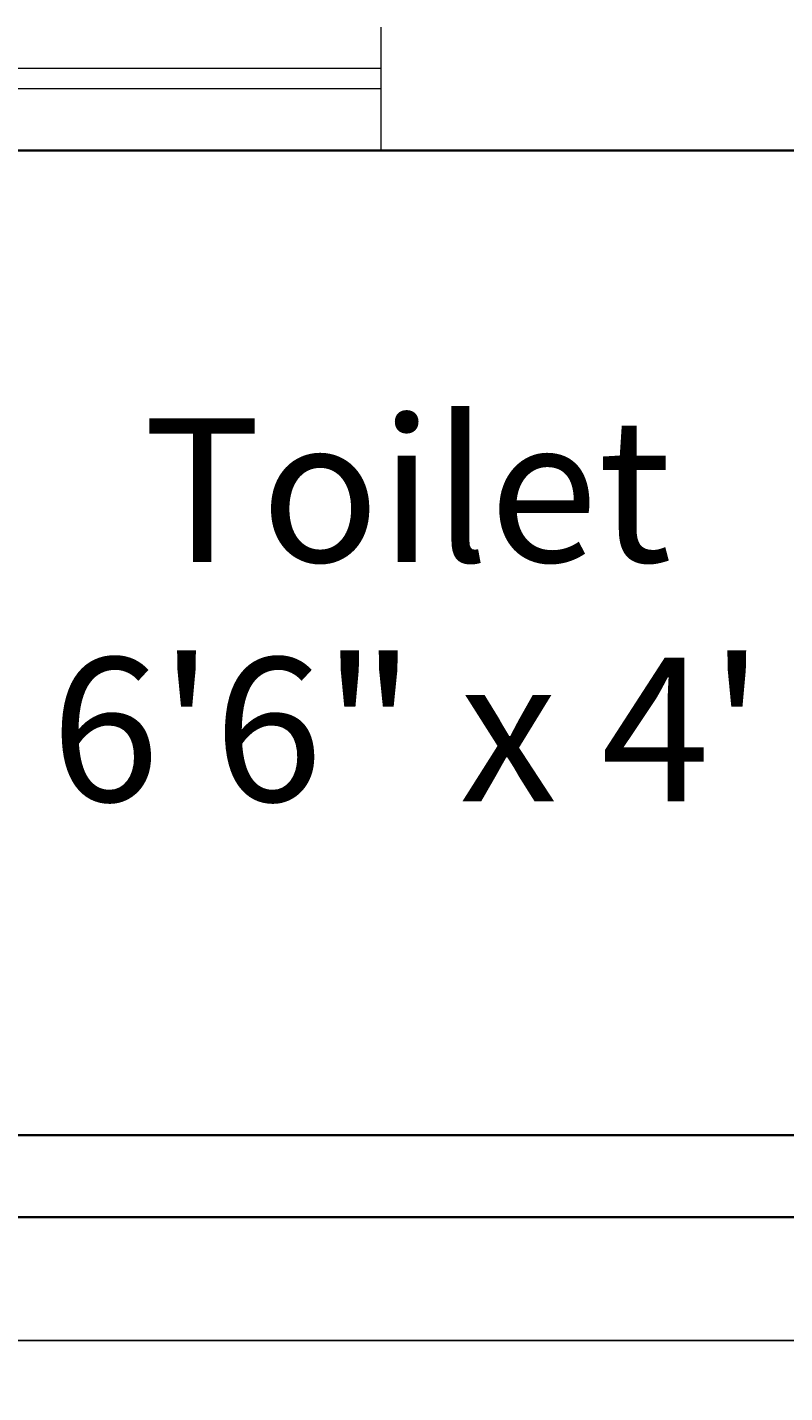
# Model space of a CAD drawing. Units: feet. Extents: x 105 to 1094, y -88 to 588.
# Tile 9 of 59: x 324 to 361, y 138 to 204. Entities that reach past the tile are written whole.
import ezdxf

# ---------------------------------------------------------------- set-up
doc = ezdxf.new("R2010")
doc.units = ezdxf.units.FT
doc.header["$MEASUREMENT"] = 0
for name, color, linetype, lineweight in [('A-ANNO-DIMS', 2, 'Continuous', 18), ('A-AREA-IDEN', 7, 'Continuous', 18), ('A-GLAZ', 4, 'Continuous', 18), ('A-WALL', 7, 'Continuous', 35)]:
    doc.layers.add(name, color=color, linetype=linetype, lineweight=lineweight)
doc.styles.get("Standard").update_dxf_attribs({"font": 'arial.ttf'})
doc.dimstyles.get("Standard").update_dxf_attribs({"dimtxt": 0.18, "dimasz": 0.18, "dimexe": 0.18, "dimexo": 0.0625, "dimgap": 0.09, "dimtad": 0, "dimtih": 1, "dimtoh": 1, "dimdec": 4, "dimzin": 0, "dimdsep": 46, "dimtxsty": 'Standard', "dimcen": 0.09, "dimadec": 0, "dimazin": 0, "dimtfac": 1, "dimtdec": 4, "dimtofl": 0, "dimtmove": 0, "dimatfit": 3, "dimfxl": 1, "dimtolj": 1, "dimtzin": 0, "dimarcsym": 0})

# ---------------------------------------------------------------- blocks, each defined once
blk = doc.blocks.new('VENT-TRANSVERSE')
for p, q in [((0, 0), (0, 6)), ((18, 0), (18, 6)), ((0, 3), (18, 3)), ((0, 2), (18, 2))]:
    blk.add_line(p, q)
blk = doc.blocks.new('*D20')
at = {"layer": 'A-ANNO-DIMS', "color": 0, "lineweight": -2, "transparency": 16777216}
for p, q in [((150.688, 276.019), (150.688, -88.149)), ((1048.688, 276.019), (1048.688, -88.149)), ((150.868, -87.969), (599.399, -87.969)), ((1048.508, -87.969), (599.977, -87.969))]:
    blk.add_line(p, q, dxfattribs=at)
at = {"layer": 'A-ANNO-DIMS', "color": 0, "transparency": 16777216}
for points in [[(150.868, -87.939), (150.868, -87.999), (150.688, -87.969)], [(1048.508, -87.939), (1048.508, -87.999), (1048.688, -87.969)]]:
    blk.add_solid(points, dxfattribs=at)
at = {"layer": 'Defpoints', "color": 0, "transparency": 16777216}
for p in [(150.688, 276.081), (1048.688, 276.081), (1048.688, -87.969)]:
    blk.add_point(p, dxfattribs=at)
at = {"layer": 'A-ANNO-DIMS', "color": 0, "transparency": 16777216, "insert": (599.688, -87.969), "char_height": 0.18, "attachment_point": 5}
blk.add_mtext('\\A1;898', dxfattribs=at)
blk = doc.blocks.new('*D21')
at = {"layer": 'A-ANNO-DIMS', "color": 0, "lineweight": -2, "transparency": 16777216}
for p, q in [((849.626, 543.081), (105.458, 543.081)), ((105.638, 542.901), (105.638, 250.263)), ((105.638, -42.739), (105.638, 249.899)), ((849.626, -42.919), (105.458, -42.919))]:
    blk.add_line(p, q, dxfattribs=at)
at = {"layer": 'A-ANNO-DIMS', "color": 0, "transparency": 16777216}
for points in [[(105.608, 542.901), (105.668, 542.901), (105.638, 543.081)], [(105.608, -42.739), (105.668, -42.739), (105.638, -42.919)]]:
    blk.add_solid(points, dxfattribs=at)
at = {"layer": 'Defpoints', "color": 0, "transparency": 16777216}
for p in [(105.638, 543.081), (849.688, 543.081), (849.688, -42.919)]:
    blk.add_point(p, dxfattribs=at)
at = {"layer": 'A-ANNO-DIMS', "color": 0, "transparency": 16777216, "insert": (105.638, 250.081), "char_height": 0.18, "attachment_point": 5}
blk.add_mtext('\\A1;586', dxfattribs=at)
blk = doc.blocks.new('*D39')
at = {"layer": 'A-ANNO-DIMS', "color": 0, "lineweight": -2, "transparency": 16777216}
for p, q in [((294.688, 204.144), (294.688, 588.311)), ((370.688, 204.144), (370.688, 588.311)), ((294.868, 588.131), (332.47, 588.131)), ((370.508, 588.131), (332.906, 588.131))]:
    blk.add_line(p, q, dxfattribs=at)
at = {"layer": 'A-ANNO-DIMS', "color": 0, "transparency": 16777216}
for points in [[(294.868, 588.161), (294.868, 588.101), (294.688, 588.131)], [(370.508, 588.161), (370.508, 588.101), (370.688, 588.131)]]:
    blk.add_solid(points, dxfattribs=at)
at = {"layer": 'Defpoints', "color": 0, "transparency": 16777216}
for p in [(370.688, 588.131), (294.688, 204.081), (370.688, 204.081)]:
    blk.add_point(p, dxfattribs=at)
at = {"layer": 'A-ANNO-DIMS', "color": 0, "transparency": 16777216, "insert": (332.688, 588.131), "char_height": 0.18, "attachment_point": 5}
blk.add_mtext('\\A1;76', dxfattribs=at)
blk = doc.blocks.new('*D46')
at = {"layer": 'A-ANNO-DIMS', "color": 0, "lineweight": -2, "transparency": 16777216}
for p, q in [((580.626, 206.081), (105.458, 206.081)), ((105.638, 205.901), (105.638, 173.263)), ((105.638, 140.261), (105.638, 172.899)), ((580.626, 140.081), (105.458, 140.081))]:
    blk.add_line(p, q, dxfattribs=at)
at = {"layer": 'A-ANNO-DIMS', "color": 0, "transparency": 16777216}
for points in [[(105.608, 205.901), (105.668, 205.901), (105.638, 206.081)], [(105.608, 140.261), (105.668, 140.261), (105.638, 140.081)]]:
    blk.add_solid(points, dxfattribs=at)
at = {"layer": 'Defpoints', "color": 0, "transparency": 16777216}
for p in [(580.688, 206.081), (105.638, 140.081), (580.688, 140.081)]:
    blk.add_point(p, dxfattribs=at)
at = {"layer": 'A-ANNO-DIMS', "color": 0, "transparency": 16777216, "insert": (105.638, 173.081), "char_height": 0.18, "attachment_point": 5}
blk.add_mtext('\\A1;66', dxfattribs=at)

msp = doc.modelspace()

# ---------------------------------------------------------------- linework, layer by layer
at = {"layer": 'A-WALL'}
for p, q in [((370.6883, 198.0812), (292.6883, 198.0812)), ((370.6883, 150.0812), (288.6883, 150.0812)), ((374.6883, 146.0812), (288.6883, 146.0812))]:
    msp.add_line(p, q, dxfattribs=at)

# ---------------------------------------------------------------- block references
at = {"layer": 'A-GLAZ', "rotation": 180}
msp.add_blockref('VENT-TRANSVERSE', (341.6886, 204.0813), dxfattribs=at)

# ---------------------------------------------------------------- texts
at = {"layer": 'A-AREA-IDEN', "insert": (392.1604, 166.3548), "char_height": 7, "attachment_point": 9}
msp.add_mtext_dynamic_manual_height_columns('\\pxqc;Toilet \\P6\'6" x 4\'', width=98.34246, gutter_width=1, heights=[0], dxfattribs=at)

# ---------------------------------------------------------------- dimensions: what is measured, and where the dimension line sits
at = {"layer": 'A-ANNO-DIMS'}
for base, p1, p2, picture, middle in [((370.6883, 588.1312), (294.6883, 204.0812), (370.6883, 204.0812), '*D39', (332.6883, 588.1312)), ((1048.6883, -87.9688), (150.6883, 276.0812), (1048.6883, 276.0812), '*D20', (599.6883, -87.9688))]:
    dim = msp.add_linear_dim(base=base, p1=p1, p2=p2, dimstyle='Standard', override={"dimdec": 0, "dimlfac": 1, "dimrnd": 0, "dimzin": 0, "dimdsep": 46, "dimlunit": 2}, dxfattribs=at)
    dim.commit()
    dim.dimension.update_dxf_attribs({"geometry": picture, "text_midpoint": middle})
for base, p1, p2, picture, middle in [((105.6383, 543.0812), (849.6883, -42.9188), (849.6883, 543.0812), '*D21', (105.6383, 250.0812)), ((105.6383, 140.0812), (580.6883, 206.0812), (580.6883, 140.0812), '*D46', (105.6383, 173.0812))]:
    dim = msp.add_linear_dim(base=base, p1=p1, p2=p2, angle=90, dimstyle='Standard', override={"dimdec": 0, "dimlfac": 1, "dimrnd": 0, "dimzin": 0, "dimdsep": 46, "dimlunit": 2}, dxfattribs=at)
    dim.commit()
    dim.dimension.update_dxf_attribs({"geometry": picture, "text_midpoint": middle})

doc.saveas('drawing.dxf')
